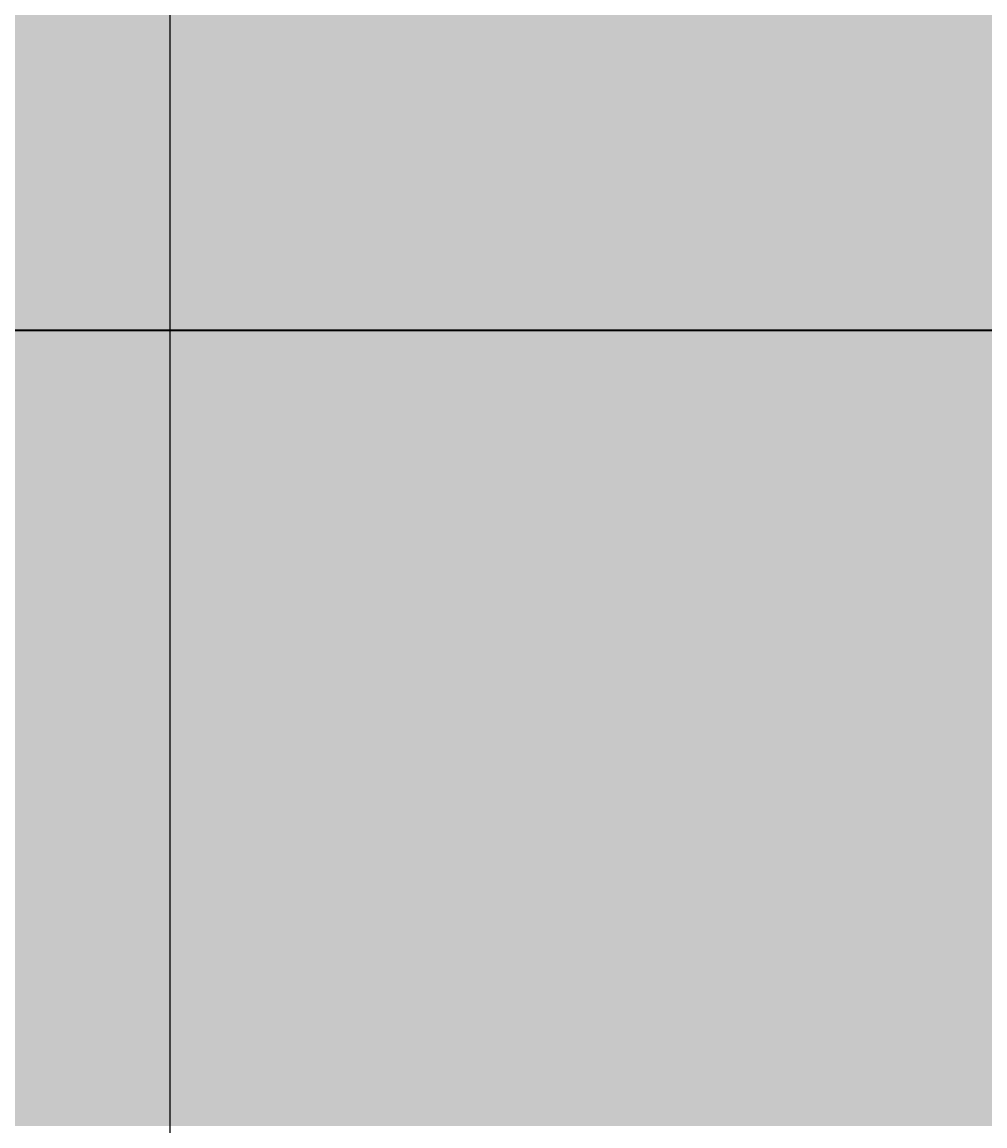
# Model space of a CAD drawing. Units: feet. Extents: x 2695 to 2912, y 795 to 1139.
# Tile 67 of 83: x 2805 to 2840, y 1021 to 1062. Entities that reach past the tile are written whole.
import ezdxf

# ---------------------------------------------------------------- set-up
doc = ezdxf.new("R2010")
doc.units = ezdxf.units.FT
for name, color, linetype, lineweight in [('A-ANNO-DIMS', 2, 'Continuous', 18), ('A-ELEV', 7, 'Continuous', 35), ('A-ELEV-PATT', 252, 'Continuous', 13)]:
    doc.layers.add(name, color=color, linetype=linetype, lineweight=lineweight)
doc.styles.get("Standard").update_dxf_attribs({"font": 'arial.ttf'})
doc.dimstyles.get("Standard").update_dxf_attribs({"dimtxt": 0.18, "dimasz": 0.18, "dimexe": 0.18, "dimexo": 0.0625, "dimgap": 0.09, "dimtad": 0, "dimtih": 1, "dimtoh": 1, "dimdec": 1, "dimzin": 0, "dimdsep": 46, "dimlunit": 3, "dimtxsty": 'Standard', "dimcen": 0.09, "dimadec": 0, "dimazin": 0, "dimtfac": 1, "dimtdec": 1, "dimtofl": 0, "dimtmove": 0, "dimatfit": 3, "dimfxl": 1, "dimtolj": 1, "dimtzin": 0, "dimarcsym": 0})

# ---------------------------------------------------------------- blocks, each defined once
blk = doc.blocks.new('*D10')
at = {"layer": 'A-ANNO-DIMS', "color": 0, "lineweight": -2, "transparency": 16777216}
for p, q in [((2778.034, 1020.886), (2778.034, 1138.886)), ((2778.214, 1138.706), (2810.411, 1138.706)), ((2843.395, 1138.706), (2811.198, 1138.706)), ((2843.575, 1020.886), (2843.575, 1138.886))]:
    blk.add_line(p, q, dxfattribs=at)
at = {"layer": 'A-ANNO-DIMS', "color": 0, "transparency": 16777216}
for points in [[(2778.214, 1138.736), (2778.214, 1138.676), (2778.034, 1138.706)], [(2843.395, 1138.736), (2843.395, 1138.676), (2843.575, 1138.706)]]:
    blk.add_solid(points, dxfattribs=at)
at = {"layer": 'Defpoints', "color": 0, "transparency": 16777216}
for p in [(2843.575, 1138.706), (2778.034, 1020.824), (2843.575, 1020.824)]:
    blk.add_point(p, dxfattribs=at)
at = {"layer": 'A-ANNO-DIMS', "color": 0, "transparency": 16777216, "insert": (2810.805, 1138.706), "char_height": 0.18, "attachment_point": 5}
blk.add_mtext('\\A1;65.54', dxfattribs=at)
blk = doc.blocks.new('*D49')
at = {"layer": 'A-ANNO-DIMS', "color": 0, "lineweight": -2, "transparency": 16777216}
for p, q in [((2772.522, 972.03), (2772.522, 1138.886)), ((2772.702, 1138.706), (2790.888, 1138.706)), ((2809.861, 1138.706), (2791.674, 1138.706)), ((2810.041, 972.03), (2810.041, 1138.886))]:
    blk.add_line(p, q, dxfattribs=at)
at = {"layer": 'A-ANNO-DIMS', "color": 0, "transparency": 16777216}
for points in [[(2772.702, 1138.736), (2772.702, 1138.676), (2772.522, 1138.706)], [(2809.861, 1138.736), (2809.861, 1138.676), (2810.041, 1138.706)]]:
    blk.add_solid(points, dxfattribs=at)
at = {"layer": 'Defpoints', "color": 0, "transparency": 16777216}
for p in [(2810.041, 1138.706), (2772.522, 971.967), (2810.041, 971.967)]:
    blk.add_point(p, dxfattribs=at)
at = {"layer": 'A-ANNO-DIMS', "color": 0, "transparency": 16777216, "insert": (2791.281, 1138.706), "char_height": 0.18, "attachment_point": 5}
blk.add_mtext('\\A1;37.52', dxfattribs=at)
blk = doc.blocks.new('*D50')
at = {"layer": 'A-ANNO-DIMS', "color": 0, "lineweight": -2, "transparency": 16777216}
for p, q in [((2810.041, 972.03), (2810.041, 1138.886)), ((2810.221, 1138.706), (2848.721, 1138.706)), ((2888.008, 1138.706), (2849.508, 1138.706)), ((2888.188, 972.03), (2888.188, 1138.886))]:
    blk.add_line(p, q, dxfattribs=at)
at = {"layer": 'A-ANNO-DIMS', "color": 0, "transparency": 16777216}
for points in [[(2810.221, 1138.736), (2810.221, 1138.676), (2810.041, 1138.706)], [(2888.008, 1138.736), (2888.008, 1138.676), (2888.188, 1138.706)]]:
    blk.add_solid(points, dxfattribs=at)
at = {"layer": 'Defpoints', "color": 0, "transparency": 16777216}
for p in [(2888.188, 1138.706), (2810.041, 971.967), (2888.188, 971.967)]:
    blk.add_point(p, dxfattribs=at)
at = {"layer": 'A-ANNO-DIMS', "color": 0, "transparency": 16777216, "insert": (2849.114, 1138.706), "char_height": 0.18, "attachment_point": 5}
blk.add_mtext('\\A1;78.15', dxfattribs=at)

msp = doc.modelspace()

# ---------------------------------------------------------------- hatches: boundary and pattern name
at = {"layer": 'A-ELEV-PATT'}
h = msp.add_hatch(color=256, dxfattribs=at)
h.set_gradient(color1=(255, 255, 255), tint=1)
h.paths.add_polyline_path([(2770.6361, 1122.9306), (2710.6361, 1122.9306), (2710.6361, 1118.4096), (2770.6361, 1118.4096)])
h.paths.add_polyline_path([(2890.6361, 1107.8588), (2770.6361, 1107.8588), (2770.6361, 1103.3378), (2890.6361, 1103.3378)])
h.paths.add_polyline_path([(2890.6361, 1062.9306), (2710.6361, 1062.9306), (2710.6361, 1056.9306), (2710.6361, 936.9306), (2710.6361, 924.3105), (2716.5358, 924.3105), (2890.6361, 924.3105), (2890.6361, 936.9306), (2715.8852, 936.9306), (2715.8852, 1050.3105), (2890.6361, 1050.3105)])
h.paths.add_polyline_path([(2716.5358, 924.3105), (2710.6361, 924.3105), (2710.6361, 810.9306), (2716.5358, 810.9306)])
h = msp.add_hatch(color=256, dxfattribs=at)
h.set_gradient(color1=(147, 149, 152), color2=(147, 149, 152), tint=1)
h.paths.add_polyline_path([(2770.6361, 1118.4096), (2710.6361, 1118.4096), (2710.6361, 1062.9306), (2770.6361, 1062.9306)])
h.paths.add_polyline_path([(2890.6361, 1103.3378), (2770.6361, 1103.3378), (2770.6361, 1062.9306), (2890.6361, 1062.9306)])
h.paths.add_polyline_path([(2730.7081, 1048.1052), (2755.1125, 1048.1052), (2755.1125, 936.9306), (2770.6361, 936.9306), (2770.6361, 1050.3105), (2715.8852, 1050.3105), (2715.8852, 936.9306), (2730.7081, 936.9306)])
h.paths.add_polyline_path([(2890.6361, 1050.3105), (2770.6361, 1050.3105), (2770.6361, 971.9673), (2778.0341, 971.9673), (2778.0341, 1020.8235), (2843.575, 1020.8235), (2843.575, 971.9673), (2890.6361, 971.9673)])
h.paths.add_polyline_path([(2888.1882, 970.7156), (2843.575, 970.7156), (2843.575, 964.8267), (2888.1882, 964.8267)])
h.paths.add_polyline_path([(2888.1882, 964.1328), (2843.575, 964.1328), (2843.575, 956.614), (2888.1882, 956.614)])
h.paths.add_polyline_path([(2888.1882, 955.9202), (2843.575, 955.9202), (2843.575, 949.2892), (2888.1882, 949.2892)])
h.paths.add_polyline_path([(2888.1882, 948.5954), (2843.575, 948.5954), (2843.575, 941.3507), (2888.1882, 941.3507)])
h.paths.add_polyline_path([(2888.1882, 940.6569), (2843.575, 940.6569), (2843.575, 936.9306), (2888.1882, 936.9306)])
h.paths.add_polyline_path([(2890.6361, 970.7156), (2888.9368, 970.7156), (2888.9368, 964.8267), (2890.6361, 964.8267)])
h.paths.add_polyline_path([(2890.6361, 964.1328), (2888.9368, 964.1328), (2888.9368, 956.614), (2890.6361, 956.614)])
h.paths.add_polyline_path([(2890.6361, 955.9202), (2888.9368, 955.9202), (2888.9368, 949.2892), (2890.6361, 949.2892)])
h.paths.add_polyline_path([(2890.6361, 940.6569), (2888.9368, 940.6569), (2888.9368, 936.9306), (2890.6361, 936.9306)])
h.paths.add_polyline_path([(2890.6361, 948.5954), (2888.9368, 948.5954), (2888.9368, 941.3507), (2890.6361, 941.3507)])
h.paths.add_polyline_path([(2772.5216, 970.7156), (2770.6361, 970.7156), (2770.6361, 964.8267), (2772.5216, 964.8267)])
h.paths.add_polyline_path([(2772.5216, 964.1328), (2770.6361, 964.1328), (2770.6361, 956.614), (2772.5216, 956.614)])
h.paths.add_polyline_path([(2772.5216, 955.9202), (2770.6361, 955.9202), (2770.6361, 949.2892), (2772.5216, 949.2892)])
h.paths.add_polyline_path([(2772.5216, 948.5954), (2770.6361, 948.5954), (2770.6361, 941.3507), (2772.5216, 941.3507)])
h.paths.add_polyline_path([(2772.5216, 940.6569), (2770.6361, 940.6569), (2770.6361, 936.9306), (2772.5216, 936.9306)])
h.paths.add_polyline_path([(2778.0341, 940.6569), (2773.2702, 940.6569), (2773.2702, 936.9306), (2778.0341, 936.9306)])
h.paths.add_polyline_path([(2778.0341, 970.7156), (2773.2702, 970.7156), (2773.2702, 964.8267), (2778.0341, 964.8267)])
h.paths.add_polyline_path([(2778.0341, 964.1328), (2773.2702, 964.1328), (2773.2702, 956.614), (2778.0341, 956.614)])
h.paths.add_polyline_path([(2778.0341, 955.9202), (2773.2702, 955.9202), (2773.2702, 949.2892), (2778.0341, 949.2892)])
h.paths.add_polyline_path([(2778.0341, 948.5954), (2773.2702, 948.5954), (2773.2702, 941.3507), (2778.0341, 941.3507)])
h.paths.add_polyline_path([(2810.0407, 940.6569), (2780.0341, 940.6569), (2780.0341, 936.9306), (2810.0407, 936.9306)])
h.paths.add_polyline_path([(2890.6361, 924.3105), (2770.6361, 924.3105), (2770.6361, 810.9306), (2773.5029, 810.9306), (2773.5029, 905.5143), (2805.9398, 905.5143), (2838.3767, 905.5143), (2838.3767, 810.9306), (2890.6361, 810.9306)])

# ---------------------------------------------------------------- linework, layer by layer
at = {"layer": 'A-ELEV'}
msp.add_line((2890.6361, 1050.3105), (2715.8852, 1050.3105), dxfattribs=at)
msp.add_lwpolyline([(2890.6361, 1050.3105), (2715.8852, 1050.3105)], dxfattribs=at)

# ---------------------------------------------------------------- dimensions: what is measured, and where the dimension line sits
at = {"layer": 'A-ANNO-DIMS'}
for base, p1, p2, picture, middle in [((2810.0407, 1138.7056), (2772.5216, 971.9673), (2810.0407, 971.9673), '*D49', (2791.2811, 1138.7056)), ((2843.575, 1138.7056), (2778.0341, 1020.8235), (2843.575, 1020.8235), '*D10', (2810.8045, 1138.7056)), ((2888.1882, 1138.7056), (2810.0407, 971.9673), (2888.1882, 971.9673), '*D50', (2849.1144, 1138.7056))]:
    dim = msp.add_linear_dim(base=base, p1=p1, p2=p2, dimstyle='Standard', override={"dimdec": 2, "dimlfac": 1, "dimrnd": 0, "dimzin": 0, "dimdsep": 46, "dimlunit": 2}, dxfattribs=at)
    dim.commit()
    dim.dimension.update_dxf_attribs({"geometry": picture, "text_midpoint": middle})

doc.saveas('drawing.dxf')
